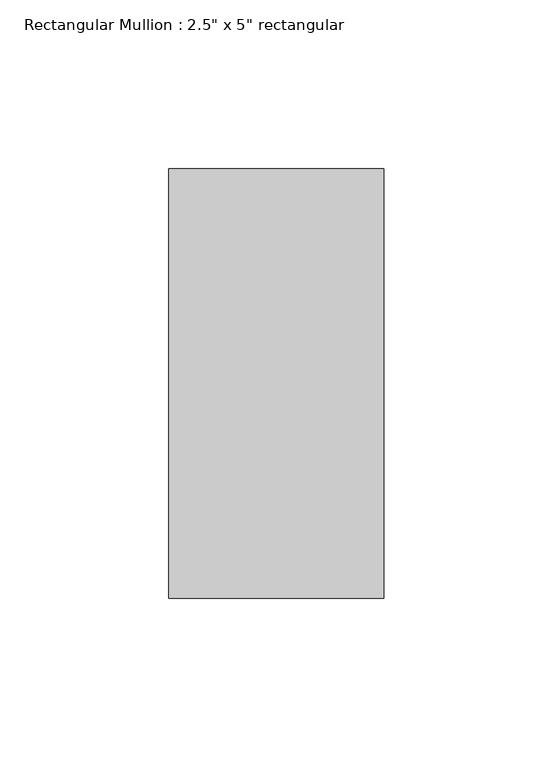
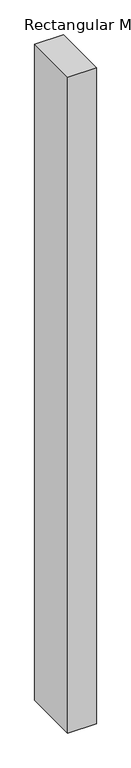
"""IFC4 building model written with IfcOpenShell, lengths in millimetres: member geometry."""

from ifc_helpers import new_model, si_unit, frame, origin, place, context, project, spatial, polyline, outline, extrude, source, transform, mapped, element, save


def member_b41a733a(model_context):
    return source(origin(), model_context, "Body", "SweptSolid", [
        extrude(outline(polyline([(0.0, 63.5), (0.0, -63.5), (-63.5, -63.5), (-63.5, 63.5), (0.0, 63.5)])), frame((0.0, 0.0, -1539.658794), z_axis=(0.0, 0.0, 1.0), x_axis=(1.0, 0.0, 0.0)), (0.0, 0.0, 1.0), 1539.658794),
    ])


if __name__ == "__main__":
    model = new_model("IFC4")
    model_context = context("Model", 3, world=origin())
    ifc_project = project(units=[si_unit("LENGTHUNIT", "METRE", prefix="MILLI")], contexts=[model_context])
    site = spatial("IfcSite", under=ifc_project)
    building = spatial("IfcBuilding", under=site)
    placement = place(None, origin())
    member_shape = member_b41a733a(model_context)
    element("IfcMember", 1, ObjectType="Rectangular Mullion : 2.5\" x 5\" rectangular", at=placement, inside=building, context=model_context, shape_type="MappedRepresentation", body=[
        mapped(member_shape, transform((0.0, 0.0, 0.0), x_axis=(1.0, 0.0, 0.0), y_axis=(0.0, 1.0, 0.0), z_axis=(0.0, 0.0, 1.0))),
    ])
    save(model, "model.ifc")

# Revit data of these elements
# Type "Rectangular Mullion : 2.5\" x 5\" rectangular"
#   built-in parameter 1007304 = 0.416667 (stored number, unit not read)
#   built-in parameter 1007301 = 0.104167 (stored number, unit not read)
#   built-in parameter 1007300 = 0.104167 (stored number, unit not read)
# Element 1 (IfcMember, "Rectangular Mullion : 2.5\" x 5\" rectangular")
#   Materials on its faces: "Aluminum"
# Materials
#   "Aluminum": class "Metal", colour RGB 247 247 247, transparency 0, Description = "Aluminum 6061", Cost = 0
